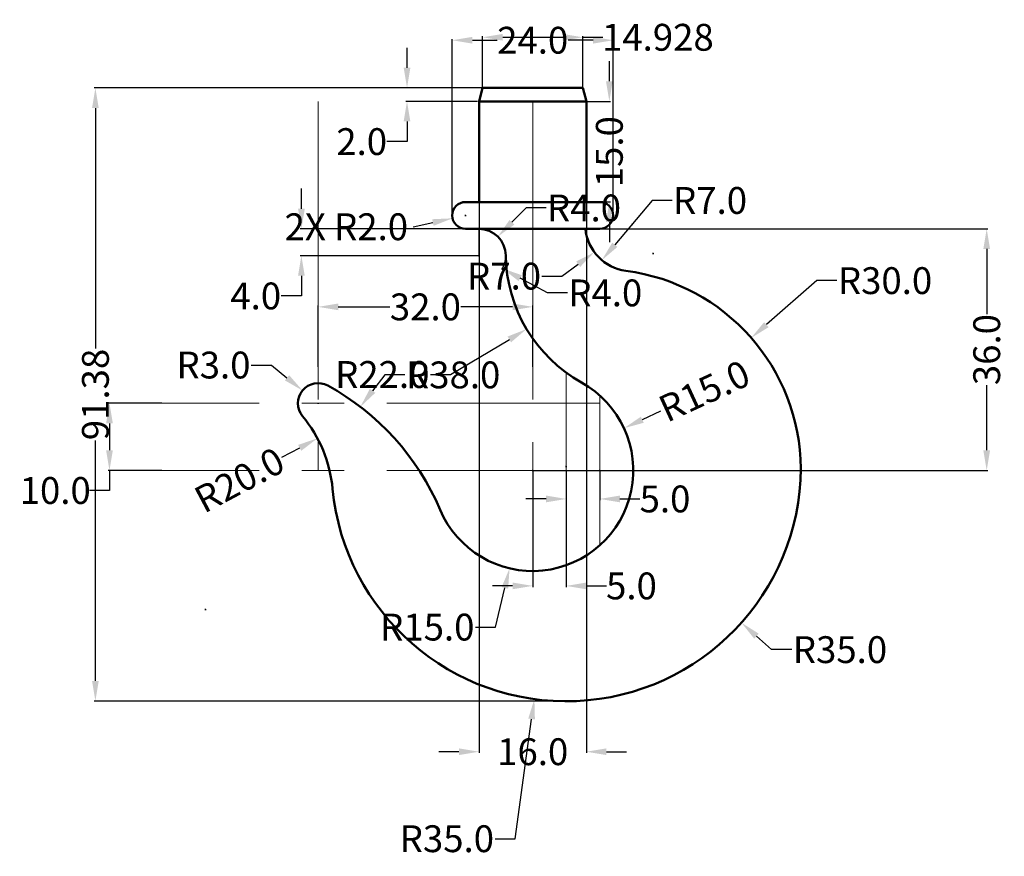
# Model space of a CAD drawing. Units: millimetres. Extents: x 373 to 520, y 647 to 772.
import ezdxf

# ---------------------------------------------------------------- set-up
doc = ezdxf.new("R2010")
doc.units = ezdxf.units.MM
doc.header["$MEASUREMENT"] = 0
doc.linetypes.add('CENTER', pattern=[50.8, 31.75, -6.35, 6.35, -6.35])
for name, color, linetype, lineweight in [('M-CNTR', 32, 'CENTER', 18), ('M-CONS', 8, 'Continuous', 13), ('M-DIMS', 2, 'Continuous', 25), ('M-OUTL', 7, 'Continuous', 50)]:
    doc.layers.add(name, color=color, linetype=linetype, lineweight=lineweight)
doc.styles.get("Standard").update_dxf_attribs({"font": 'arial.ttf'})
doc.dimstyles.get("Standard").update_dxf_attribs({"dimtxt": 4, "dimasz": 3, "dimexe": 0.18, "dimexo": 0.0625, "dimgap": 0.09, "dimtad": 0, "dimtoh": 1, "dimdec": 1, "dimzin": 0, "dimdsep": 46, "dimtxsty": 'Standard', "dimcen": 0.09, "dimadec": 0, "dimazin": 0, "dimtfac": 1, "dimtdec": 1, "dimtofl": 0, "dimtmove": 0, "dimatfit": 3, "dimfxl": 1, "dimtolj": 1, "dimtzin": 0, "dimarcsym": 0})

# ---------------------------------------------------------------- blocks, each defined once
blk = doc.blocks.new('*D1')
at = {"layer": 'Defpoints', "color": 0, "transparency": 16777216}
for p in [(482.23, 724.42), (459.65, 704.68)]:
    blk.add_point(p, dxfattribs=at)
at = {"layer": 'M-DIMS', "color": 0, "lineweight": -2, "transparency": 16777216}
for p, q in [((492, 732.96), (484.49, 726.4)), ((495, 732.96), (492, 732.96)), ((459.65, 704.59), (459.65, 704.77)), ((459.56, 704.68), (459.74, 704.68))]:
    blk.add_line(p, q, dxfattribs=at)
at = {"layer": 'M-DIMS', "color": 0, "transparency": 16777216}
blk.add_solid([(484.16, 726.77), (484.82, 726.02), (482.23, 724.42)], dxfattribs=at)
at = {"layer": 'M-DIMS', "color": 0, "transparency": 16777216, "insert": (502.19, 732.96), "char_height": 4, "attachment_point": 5}
blk.add_mtext('\\A1;R30.0', dxfattribs=at)
blk = doc.blocks.new('*D2')
at = {"layer": 'Defpoints', "color": 0, "transparency": 16777216}
for p in [(454.65, 705.26), (480.78, 681.97)]:
    blk.add_point(p, dxfattribs=at)
at = {"layer": 'M-DIMS', "color": 0, "lineweight": -2, "transparency": 16777216}
for p, q in [((454.56, 705.26), (454.74, 705.26)), ((454.65, 705.17), (454.65, 705.35)), ((485.27, 677.96), (483.01, 679.98)), ((488.27, 677.96), (485.27, 677.96))]:
    blk.add_line(p, q, dxfattribs=at)
at = {"layer": 'M-DIMS', "color": 0, "transparency": 16777216}
blk.add_solid([(483.35, 680.35), (482.68, 679.6), (480.78, 681.97)], dxfattribs=at)
at = {"layer": 'M-DIMS', "color": 0, "transparency": 16777216, "insert": (495.47, 677.96), "char_height": 4, "attachment_point": 5}
blk.add_mtext('\\A1;R35.0', dxfattribs=at)
blk = doc.blocks.new('*D3')
at = {"layer": 'Defpoints', "color": 0, "transparency": 16777216}
for p in [(441.64, 736.68), (445.15, 734.77)]:
    blk.add_point(p, dxfattribs=at)
at = {"layer": 'M-DIMS', "color": 0, "lineweight": -2, "transparency": 16777216}
for p, q in [((441.55, 736.68), (441.73, 736.68)), ((441.64, 736.59), (441.64, 736.77)), ((451.84, 731.13), (447.79, 733.33)), ((454.84, 731.13), (451.84, 731.13))]:
    blk.add_line(p, q, dxfattribs=at)
blk.add_arc((441.64, 736.68), 4, 328.9016, 359.8455, dxfattribs=at)
at = {"layer": 'M-DIMS', "color": 0, "transparency": 16777216}
blk.add_solid([(448.03, 733.77), (447.55, 732.89), (445.15, 734.77)], dxfattribs=at)
at = {"layer": 'M-DIMS', "color": 0, "transparency": 16777216, "insert": (460.47, 731.13), "char_height": 4, "attachment_point": 5}
blk.add_mtext('\\A1;R4.0', dxfattribs=at)
blk = doc.blocks.new('*D4')
at = {"layer": 'Defpoints', "color": 0, "transparency": 16777216}
for p in [(464.48, 741.36), (459.96, 736.01)]:
    blk.add_point(p, dxfattribs=at)
at = {"layer": 'M-DIMS', "color": 0, "lineweight": -2, "transparency": 16777216}
for p, q in [((467.47, 744.91), (461.9, 738.3)), ((470.47, 744.91), (467.47, 744.91))]:
    blk.add_line(p, q, dxfattribs=at)
at = {"layer": 'M-DIMS', "color": 0, "transparency": 16777216}
blk.add_solid([(461.51, 738.62), (462.28, 737.98), (459.96, 736.01)], dxfattribs=at)
at = {"layer": 'M-DIMS', "color": 0, "transparency": 16777216, "insert": (476.1, 744.91), "char_height": 4, "attachment_point": 5}
blk.add_mtext('\\A1;R7.0', dxfattribs=at)
blk = doc.blocks.new('*D5')
at = {"layer": 'Defpoints', "color": 0, "transparency": 16777216}
for p in [(441.46, 761.68), (430.91, 759.68), (441.46, 759.68)]:
    blk.add_point(p, dxfattribs=at)
at = {"layer": 'M-DIMS', "color": 0, "lineweight": -2, "transparency": 16777216}
for p, q in [((430.91, 764.68), (430.91, 767.68)), ((441.4, 761.68), (430.73, 761.68)), ((441.4, 759.68), (430.73, 759.68)), ((430.91, 756.68), (430.91, 753.68)), ((430.91, 753.68), (427.91, 753.68))]:
    blk.add_line(p, q, dxfattribs=at)
at = {"layer": 'M-DIMS', "color": 0, "transparency": 16777216}
for points in [[(430.41, 764.68), (431.41, 764.68), (430.91, 761.68)], [(430.41, 756.68), (431.41, 756.68), (430.91, 759.68)]]:
    blk.add_solid(points, dxfattribs=at)
at = {"layer": 'M-DIMS', "color": 0, "transparency": 16777216, "insert": (424.15, 753.68), "char_height": 4, "attachment_point": 5}
blk.add_mtext('\\A1;2.0', dxfattribs=at)
blk = doc.blocks.new('*D6')
at = {"layer": 'Defpoints', "color": 0, "transparency": 16777216}
for p in [(457.65, 759.68), (461.08, 759.68), (457.65, 744.68)]:
    blk.add_point(p, dxfattribs=at)
at = {"layer": 'M-DIMS', "color": 0, "lineweight": -2, "transparency": 16777216}
for p, q in [((461.08, 762.68), (461.08, 765.68)), ((457.71, 759.68), (461.26, 759.68)), ((457.71, 744.68), (461.26, 744.68)), ((461.08, 741.68), (461.08, 738.68))]:
    blk.add_line(p, q, dxfattribs=at)
at = {"layer": 'M-DIMS', "color": 0, "transparency": 16777216}
for points in [[(460.58, 762.68), (461.58, 762.68), (461.08, 759.68)], [(460.58, 741.68), (461.58, 741.68), (461.08, 744.68)]]:
    blk.add_solid(points, dxfattribs=at)
at = {"layer": 'M-DIMS', "color": 0, "transparency": 16777216, "insert": (461.08, 752.18), "char_height": 4, "attachment_point": 5, "rotation": 90}
blk.add_mtext('\\A1;15.0', dxfattribs=at)
blk = doc.blocks.new('*D7')
at = {"layer": 'Defpoints', "color": 0, "transparency": 16777216}
for p in [(461.65, 768.79), (437.65, 742.68), (461.65, 742.68)]:
    blk.add_point(p, dxfattribs=at)
at = {"layer": 'M-DIMS', "color": 0, "lineweight": -2, "transparency": 16777216}
for p, q in [((437.65, 742.74), (437.65, 768.97)), ((440.65, 768.79), (444.34, 768.79)), ((458.65, 768.79), (454.96, 768.79)), ((461.65, 742.74), (461.65, 768.97))]:
    blk.add_line(p, q, dxfattribs=at)
at = {"layer": 'M-DIMS', "color": 0, "transparency": 16777216}
for points in [[(440.65, 769.29), (440.65, 768.29), (437.65, 768.79)], [(458.65, 769.29), (458.65, 768.29), (461.65, 768.79)]]:
    blk.add_solid(points, dxfattribs=at)
at = {"layer": 'M-DIMS', "color": 0, "transparency": 16777216, "insert": (449.65, 768.79), "char_height": 4, "attachment_point": 5}
blk.add_mtext('\\A1;24.0', dxfattribs=at)
blk = doc.blocks.new('*D8')
at = {"layer": 'Defpoints', "color": 0, "transparency": 16777216}
for p in [(449.65, 704.68), (454.65, 704.68), (454.65, 687.46)]:
    blk.add_point(p, dxfattribs=at)
at = {"layer": 'M-DIMS', "color": 0, "lineweight": -2, "transparency": 16777216}
for p, q in [((449.65, 704.61), (449.65, 687.28)), ((454.65, 704.61), (454.65, 687.28)), ((446.65, 687.46), (443.65, 687.46)), ((457.65, 687.46), (460.65, 687.46))]:
    blk.add_line(p, q, dxfattribs=at)
at = {"layer": 'M-DIMS', "color": 0, "transparency": 16777216}
for points in [[(446.65, 687.96), (446.65, 686.96), (449.65, 687.46)], [(457.65, 687.96), (457.65, 686.96), (454.65, 687.46)]]:
    blk.add_solid(points, dxfattribs=at)
at = {"layer": 'M-DIMS', "color": 0, "transparency": 16777216, "insert": (464.38, 687.46), "char_height": 4, "attachment_point": 5}
blk.add_mtext('\\A1;5.0', dxfattribs=at)
blk = doc.blocks.new('*D9')
at = {"layer": 'Defpoints', "color": 0, "transparency": 16777216}
for p in [(454.65, 704.68), (459.65, 704.59), (459.65, 700.42)]:
    blk.add_point(p, dxfattribs=at)
at = {"layer": 'M-DIMS', "color": 0, "lineweight": -2, "transparency": 16777216}
for p, q in [((454.65, 704.61), (454.65, 700.24)), ((459.65, 704.52), (459.65, 700.24)), ((451.65, 700.42), (448.65, 700.42)), ((462.65, 700.42), (465.65, 700.42))]:
    blk.add_line(p, q, dxfattribs=at)
at = {"layer": 'M-DIMS', "color": 0, "transparency": 16777216}
for points in [[(451.65, 700.92), (451.65, 699.92), (454.65, 700.42)], [(462.65, 700.92), (462.65, 699.92), (459.65, 700.42)]]:
    blk.add_solid(points, dxfattribs=at)
at = {"layer": 'M-DIMS', "color": 0, "transparency": 16777216, "insert": (469.38, 700.42), "char_height": 4, "attachment_point": 5}
blk.add_mtext('\\A1;5.0', dxfattribs=at)
blk = doc.blocks.new('*D10')
at = {"layer": 'Defpoints', "color": 0, "transparency": 16777216}
for p in [(463.27, 710.97), (449.65, 704.68)]:
    blk.add_point(p, dxfattribs=at)
at = {"layer": 'M-DIMS', "color": 0, "lineweight": -2, "transparency": 16777216}
for p, q in [((468.71, 713.49), (465.99, 712.23)), ((449.65, 704.59), (449.65, 704.77)), ((449.56, 704.68), (449.74, 704.68))]:
    blk.add_line(p, q, dxfattribs=at)
at = {"layer": 'M-DIMS', "color": 0, "transparency": 16777216}
blk.add_solid([(465.78, 712.68), (466.2, 711.77), (463.27, 710.97)], dxfattribs=at)
at = {"layer": 'M-DIMS', "color": 0, "transparency": 16777216, "insert": (475.24, 716.51), "char_height": 4, "attachment_point": 5, "rotation": 24.8104}
blk.add_mtext('\\A1;R15.0', dxfattribs=at)
blk = doc.blocks.new('*D11')
at = {"layer": 'Defpoints', "color": 0, "transparency": 16777216}
for p in [(415.33, 716.58), (417.65, 714.68)]:
    blk.add_point(p, dxfattribs=at)
at = {"layer": 'M-DIMS', "color": 0, "lineweight": -2, "transparency": 16777216}
for p, q in [((407.69, 720.38), (410.69, 720.38)), ((410.69, 720.38), (413.01, 718.48)), ((417.56, 714.68), (417.74, 714.68)), ((417.65, 714.59), (417.65, 714.77))]:
    blk.add_line(p, q, dxfattribs=at)
at = {"layer": 'M-DIMS', "color": 0, "transparency": 16777216}
blk.add_solid([(413.33, 718.87), (412.69, 718.09), (415.33, 716.58)], dxfattribs=at)
at = {"layer": 'M-DIMS', "color": 0, "transparency": 16777216, "insert": (402.05, 720.38), "char_height": 4, "attachment_point": 5}
blk.add_mtext('\\A1;R3.0', dxfattribs=at)
blk = doc.blocks.new('*D12')
at = {"layer": 'Defpoints', "color": 0, "transparency": 16777216}
for p in [(417.55, 709.45), (399.9, 700.05)]:
    blk.add_point(p, dxfattribs=at)
at = {"layer": 'M-DIMS', "color": 0, "lineweight": -2, "transparency": 16777216}
blk.add_line((412.26, 706.63), (414.91, 708.04), dxfattribs=at)
at = {"layer": 'M-DIMS', "color": 0, "transparency": 16777216}
blk.add_solid([(414.67, 708.48), (415.14, 707.6), (417.55, 709.45)], dxfattribs=at)
at = {"layer": 'M-DIMS', "color": 0, "transparency": 16777216, "insert": (405.91, 703.25), "char_height": 4, "attachment_point": 5, "rotation": 28.0286}
blk.add_mtext('\\A1;R20.0', dxfattribs=at)
blk = doc.blocks.new('*D13')
at = {"layer": 'Defpoints', "color": 0, "transparency": 16777216}
for p in [(423.95, 714.15), (400.87, 683.96)]:
    blk.add_point(p, dxfattribs=at)
at = {"layer": 'M-DIMS', "color": 0, "lineweight": -2, "transparency": 16777216}
for p, q in [((427.59, 718.91), (425.77, 716.53)), ((430.59, 718.91), (427.59, 718.91)), ((400.78, 683.96), (400.96, 683.96)), ((400.87, 683.87), (400.87, 684.05))]:
    blk.add_line(p, q, dxfattribs=at)
at = {"layer": 'M-DIMS', "color": 0, "transparency": 16777216}
blk.add_solid([(425.37, 716.84), (426.17, 716.23), (423.95, 714.15)], dxfattribs=at)
at = {"layer": 'M-DIMS', "color": 0, "transparency": 16777216, "insert": (437.79, 718.91), "char_height": 4, "attachment_point": 5}
blk.add_mtext('\\A1;R38.0', dxfattribs=at)
blk = doc.blocks.new('*D14')
at = {"layer": 'Defpoints', "color": 0, "transparency": 16777216}
for p in [(394.4, 714.68), (386.54, 704.68), (394.4, 704.68)]:
    blk.add_point(p, dxfattribs=at)
at = {"layer": 'M-DIMS', "color": 0, "lineweight": -2, "transparency": 16777216}
for p, q in [((394.34, 714.68), (386.36, 714.68)), ((386.54, 711.68), (386.54, 707.68)), ((394.34, 704.68), (386.36, 704.68)), ((386.54, 704.68), (386.54, 701.68)), ((386.54, 701.68), (383.54, 701.68))]:
    blk.add_line(p, q, dxfattribs=at)
at = {"layer": 'M-DIMS', "color": 0, "transparency": 16777216}
for points in [[(386.04, 711.68), (387.04, 711.68), (386.54, 714.68)], [(386.04, 707.68), (387.04, 707.68), (386.54, 704.68)]]:
    blk.add_solid(points, dxfattribs=at)
at = {"layer": 'M-DIMS', "color": 0, "transparency": 16777216, "insert": (378.45, 701.68), "char_height": 4, "attachment_point": 5}
blk.add_mtext('\\A1;10.0', dxfattribs=at)
blk = doc.blocks.new('*D15')
at = {"layer": 'Defpoints', "color": 0, "transparency": 16777216}
for p in [(449.65, 740.68), (449.74, 704.68), (517.35, 704.68)]:
    blk.add_point(p, dxfattribs=at)
at = {"layer": 'M-DIMS', "color": 0, "lineweight": -2, "transparency": 16777216}
for p, q in [((449.71, 740.68), (517.53, 740.68)), ((517.35, 737.68), (517.35, 727.95)), ((517.35, 707.68), (517.35, 717.4)), ((449.8, 704.68), (517.53, 704.68))]:
    blk.add_line(p, q, dxfattribs=at)
at = {"layer": 'M-DIMS', "color": 0, "transparency": 16777216}
for points in [[(516.85, 737.68), (517.85, 737.68), (517.35, 740.68)], [(516.85, 707.68), (517.85, 707.68), (517.35, 704.68)]]:
    blk.add_solid(points, dxfattribs=at)
at = {"layer": 'M-DIMS', "color": 0, "transparency": 16777216, "insert": (517.35, 722.68), "char_height": 4, "attachment_point": 5, "rotation": 90}
blk.add_mtext('\\A1;36.0', dxfattribs=at)
blk = doc.blocks.new('*D16')
at = {"layer": 'Defpoints', "color": 0, "transparency": 16777216}
for p in [(417.65, 729.05), (417.65, 720.04), (449.65, 720.04)]:
    blk.add_point(p, dxfattribs=at)
at = {"layer": 'M-DIMS', "color": 0, "lineweight": -2, "transparency": 16777216}
for p, q in [((417.65, 720.11), (417.65, 729.23)), ((420.65, 729.05), (428.37, 729.05)), ((446.65, 729.05), (438.93, 729.05)), ((449.65, 720.11), (449.65, 729.23))]:
    blk.add_line(p, q, dxfattribs=at)
at = {"layer": 'M-DIMS', "color": 0, "transparency": 16777216}
for points in [[(420.65, 729.55), (420.65, 728.55), (417.65, 729.05)], [(446.65, 729.55), (446.65, 728.55), (449.65, 729.05)]]:
    blk.add_solid(points, dxfattribs=at)
at = {"layer": 'M-DIMS', "color": 0, "transparency": 16777216, "insert": (433.65, 729.05), "char_height": 4, "attachment_point": 5}
blk.add_mtext('\\A1;32.0', dxfattribs=at)
blk = doc.blocks.new('*D17')
at = {"layer": 'Defpoints', "color": 0, "transparency": 16777216}
for p in [(441.64, 740.68), (415.16, 736.68), (441.64, 736.68)]:
    blk.add_point(p, dxfattribs=at)
at = {"layer": 'M-DIMS', "color": 0, "lineweight": -2, "transparency": 16777216}
for p, q in [((415.16, 743.68), (415.16, 746.68)), ((441.57, 740.68), (414.98, 740.68)), ((441.57, 736.68), (414.98, 736.68)), ((415.16, 733.68), (415.16, 730.68)), ((415.16, 730.68), (412.16, 730.68))]:
    blk.add_line(p, q, dxfattribs=at)
at = {"layer": 'M-DIMS', "color": 0, "transparency": 16777216}
for points in [[(414.66, 743.68), (415.66, 743.68), (415.16, 740.68)], [(414.66, 733.68), (415.66, 733.68), (415.16, 736.68)]]:
    blk.add_solid(points, dxfattribs=at)
at = {"layer": 'M-DIMS', "color": 0, "transparency": 16777216, "insert": (408.35, 730.68), "char_height": 4, "attachment_point": 5}
blk.add_mtext('\\A1;4.0', dxfattribs=at)
blk = doc.blocks.new('*D18')
at = {"layer": 'Defpoints', "color": 0, "transparency": 16777216}
for p in [(442.19, 761.68), (384.44, 670.3), (456.16, 670.3)]:
    blk.add_point(p, dxfattribs=at)
at = {"layer": 'M-DIMS', "color": 0, "lineweight": -2, "transparency": 16777216}
for p, q in [((442.12, 761.68), (384.26, 761.68)), ((384.44, 758.68), (384.44, 722.83)), ((384.44, 673.3), (384.44, 709.14)), ((456.1, 670.3), (384.26, 670.3))]:
    blk.add_line(p, q, dxfattribs=at)
at = {"layer": 'M-DIMS', "color": 0, "transparency": 16777216}
for points in [[(383.94, 758.68), (384.94, 758.68), (384.44, 761.68)], [(383.94, 673.3), (384.94, 673.3), (384.44, 670.3)]]:
    blk.add_solid(points, dxfattribs=at)
at = {"layer": 'M-DIMS', "color": 0, "transparency": 16777216, "insert": (384.44, 715.99), "char_height": 4, "attachment_point": 5, "rotation": 90}
blk.add_mtext('\\A1;91.38', dxfattribs=at)
blk = doc.blocks.new('*D19')
at = {"layer": 'Defpoints', "color": 0, "transparency": 16777216}
for p in [(441.651389, 759.675544), (457.651389, 759.675544), (457.651389, 662.747036)]:
    blk.add_point(p, dxfattribs=at)
at = {"layer": 'M-DIMS', "color": 0, "lineweight": -2, "transparency": 16777216}
for p, q in [((441.651389, 759.613044), (441.651389, 662.567036)), ((457.651389, 759.613044), (457.651389, 662.567036)), ((438.651389, 662.747036), (435.651389, 662.747036)), ((460.651389, 662.747036), (463.651389, 662.747036))]:
    blk.add_line(p, q, dxfattribs=at)
at = {"layer": 'M-DIMS', "color": 0, "transparency": 16777216}
for points in [[(438.651389, 663.247036), (438.651389, 662.247036), (441.651389, 662.747036)], [(460.651389, 663.247036), (460.651389, 662.247036), (457.651389, 662.747036)]]:
    blk.add_solid(points, dxfattribs=at)
at = {"layer": 'M-DIMS', "color": 0, "transparency": 16777216, "insert": (449.651389, 662.747036), "char_height": 4, "attachment_point": 5}
blk.add_mtext('\\A1;16.0', dxfattribs=at)
blk = doc.blocks.new('*D20')
at = {"layer": 'Defpoints', "color": 0, "transparency": 16777216}
for p in [(457.12, 769.23), (442.19, 761.68), (457.12, 761.68)]:
    blk.add_point(p, dxfattribs=at)
at = {"layer": 'M-DIMS', "color": 0, "lineweight": -2, "transparency": 16777216}
for p, q in [((442.19, 761.74), (442.19, 769.41)), ((457.12, 761.74), (457.12, 769.41)), ((445.19, 769.23), (454.12, 769.23)), ((457.12, 769.23), (460.12, 769.23))]:
    blk.add_line(p, q, dxfattribs=at)
at = {"layer": 'M-DIMS', "color": 0, "transparency": 16777216}
for points in [[(445.19, 769.73), (445.19, 768.73), (442.19, 769.23)], [(454.12, 769.73), (454.12, 768.73), (457.12, 769.23)]]:
    blk.add_solid(points, dxfattribs=at)
at = {"layer": 'M-DIMS', "color": 0, "transparency": 16777216, "insert": (468.32, 769.23), "char_height": 4, "attachment_point": 5}
blk.add_mtext('\\A1;14.928', dxfattribs=at)
blk = doc.blocks.new('*D21')
at = {"layer": 'Defpoints', "color": 0, "transparency": 16777216}
for p in [(454.65, 705.26), (449.9, 670.59)]:
    blk.add_point(p, dxfattribs=at)
at = {"layer": 'M-DIMS', "color": 0, "lineweight": -2, "transparency": 16777216}
for p, q in [((454.56, 705.26), (454.74, 705.26)), ((454.65, 705.17), (454.65, 705.35)), ((447.04, 649.78), (449.49, 667.62)), ((444.04, 649.78), (447.04, 649.78))]:
    blk.add_line(p, q, dxfattribs=at)
at = {"layer": 'M-DIMS', "color": 0, "transparency": 16777216}
blk.add_solid([(448.99, 667.68), (449.98, 667.55), (449.9, 670.59)], dxfattribs=at)
at = {"layer": 'M-DIMS', "color": 0, "transparency": 16777216, "insert": (436.85, 649.78), "char_height": 4, "attachment_point": 5}
blk.add_mtext('\\A1;R35.0', dxfattribs=at)
blk = doc.blocks.new('*D22')
at = {"layer": 'Defpoints', "color": 0, "transparency": 16777216}
for p in [(449.65, 704.68), (446.2, 690.08)]:
    blk.add_point(p, dxfattribs=at)
at = {"layer": 'M-DIMS', "color": 0, "lineweight": -2, "transparency": 16777216}
for p, q in [((449.65, 704.59), (449.65, 704.77)), ((449.56, 704.68), (449.74, 704.68)), ((444.12, 681.32), (445.5, 687.16)), ((441.12, 681.32), (444.12, 681.32))]:
    blk.add_line(p, q, dxfattribs=at)
at = {"layer": 'M-DIMS', "color": 0, "transparency": 16777216}
blk.add_solid([(445.02, 687.28), (445.99, 687.04), (446.2, 690.08)], dxfattribs=at)
at = {"layer": 'M-DIMS', "color": 0, "transparency": 16777216, "insert": (433.93, 681.32), "char_height": 4, "attachment_point": 5}
blk.add_mtext('\\A1;R15.0', dxfattribs=at)
blk = doc.blocks.new('*D23')
at = {"layer": 'Defpoints', "color": 0, "transparency": 16777216}
for p in [(467.63, 737.01), (448.74, 725.74)]:
    blk.add_point(p, dxfattribs=at)
at = {"layer": 'M-DIMS', "color": 0, "lineweight": -2, "transparency": 16777216}
for p, q in [((467.63, 736.92), (467.63, 737.1)), ((467.54, 737.01), (467.72, 737.01)), ((437.41, 718.97), (446.17, 724.2)), ((434.41, 718.97), (437.41, 718.97))]:
    blk.add_line(p, q, dxfattribs=at)
at = {"layer": 'M-DIMS', "color": 0, "transparency": 16777216}
blk.add_solid([(445.91, 724.63), (446.42, 723.77), (448.74, 725.74)], dxfattribs=at)
at = {"layer": 'M-DIMS', "color": 0, "transparency": 16777216, "insert": (427.22, 718.97), "char_height": 4, "attachment_point": 5}
blk.add_mtext('\\A1;R22.0', dxfattribs=at)
blk = doc.blocks.new('*D24')
at = {"layer": 'Defpoints', "color": 0, "transparency": 16777216}
for p in [(464.48, 741.36), (458.85, 737.2)]:
    blk.add_point(p, dxfattribs=at)
at = {"layer": 'M-DIMS', "color": 0, "lineweight": -2, "transparency": 16777216}
for p, q in [((464.39, 741.36), (464.57, 741.36)), ((464.48, 741.27), (464.48, 741.45)), ((454.02, 733.63), (456.43, 735.41)), ((451.02, 733.63), (454.02, 733.63))]:
    blk.add_line(p, q, dxfattribs=at)
at = {"layer": 'M-DIMS', "color": 0, "transparency": 16777216}
blk.add_solid([(456.14, 735.82), (456.73, 735.01), (458.85, 737.2)], dxfattribs=at)
at = {"layer": 'M-DIMS', "color": 0, "transparency": 16777216, "insert": (445.38, 733.63), "char_height": 4, "attachment_point": 5}
blk.add_mtext('\\A1;R7.0', dxfattribs=at)
blk = doc.blocks.new('*D25')
at = {"layer": 'Defpoints', "color": 0, "transparency": 16777216}
for p in [(444.45, 739.52), (441.64, 736.68)]:
    blk.add_point(p, dxfattribs=at)
at = {"layer": 'M-DIMS', "color": 0, "lineweight": -2, "transparency": 16777216}
for p, q in [((448.66, 743.79), (446.55, 741.66)), ((451.66, 743.79), (448.66, 743.79)), ((441.55, 736.68), (441.73, 736.68)), ((441.64, 736.59), (441.64, 736.77))]:
    blk.add_line(p, q, dxfattribs=at)
at = {"layer": 'M-DIMS', "color": 0, "transparency": 16777216}
blk.add_solid([(446.2, 742.01), (446.91, 741.31), (444.45, 739.52)], dxfattribs=at)
at = {"layer": 'M-DIMS', "color": 0, "transparency": 16777216, "insert": (457.3, 743.79), "char_height": 4, "attachment_point": 5}
blk.add_mtext('\\A1;R4.0', dxfattribs=at)
blk = doc.blocks.new('*D26')
at = {"layer": 'Defpoints', "color": 0, "transparency": 16777216}
for p in [(437.7, 742.25), (439.65, 742.68)]:
    blk.add_point(p, dxfattribs=at)
at = {"layer": 'M-DIMS', "color": 0, "lineweight": -2, "transparency": 16777216}
for p, q in [((431.83, 740.99), (434.76, 741.62)), ((439.56, 742.68), (439.74, 742.68)), ((439.65, 742.59), (439.65, 742.77))]:
    blk.add_line(p, q, dxfattribs=at)
at = {"layer": 'M-DIMS', "color": 0, "transparency": 16777216}
blk.add_solid([(434.66, 742.11), (434.87, 741.13), (437.7, 742.25)], dxfattribs=at)
at = {"layer": 'M-DIMS', "color": 0, "transparency": 16777216, "insert": (421.86, 740.99), "char_height": 4, "attachment_point": 5}
blk.add_mtext('\\A1;2X R2.0', dxfattribs=at)

msp = doc.modelspace()

# ---------------------------------------------------------------- linework, layer by layer
at = {"layer": 'M-CNTR'}
for p, q in [((417.6514, 759.6755), (417.6514, 704.6755)), ((449.6514, 759.6755), (449.6514, 689.6755)), ((454.6514, 719.2507), (454.6514, 690.5334)), ((459.6514, 715.8559), (459.6514, 693.4952))]:
    msp.add_line(p, q, dxfattribs=at)
for points in [[(459.6514, 714.6755), (391.9947, 714.6755)], [(459.6514, 704.6755), (391.9947, 704.6755)]]:
    msp.add_lwpolyline(points, dxfattribs=at)
at = {"layer": 'M-CONS'}
msp.add_line((441.6362, 740.6755), (441.6362, 736.6755), dxfattribs=at)
at = {"layer": 'M-OUTL'}
for points in [[(441.6514, 759.6755), (457.6514, 759.6755), (457.6514, 759.6755), (457.1155, 761.6755), (442.1873, 761.6755), (441.6514, 759.6755)], [(441.6514, 759.6755), (457.6514, 759.6755), (457.6514, 744.6755), (441.6514, 744.6755)]]:
    msp.add_lwpolyline(points, close=True, dxfattribs=at)
for points in [[(439.6514, 744.6755), (459.6514, 744.6755)], [(459.6514, 740.6755), (439.6514, 740.6755)]]:
    msp.add_lwpolyline(points, dxfattribs=at)
for centre, radius, start, end in [((439.6514, 742.6755), 2, 90, 270), ((459.6514, 742.6755), 2, 270, 90), ((441.6362, 736.6755), 4, 0.74073, 90), ((464.4752, 741.3598), 7, 185.609295, 262.508911), ((467.634, 737.0117), 22, 180.74073, 240.920865), ((459.6514, 704.6755), 30, 0.540801, 82.508911), ((417.6514, 714.6755), 3, 61.342286, 219.480177), ((400.8662, 683.963), 38, 23.004419, 61.342286), ((449.6514, 704.6755), 15, 203.004419, 60.920865), ((399.899, 700.0519), 20, 5.43841, 39.480177), ((454.6514, 705.2645), 35, 185.43841, 359.499316)]:
    msp.add_arc(centre, radius, start, end, dxfattribs=at)

# ---------------------------------------------------------------- dimensions: what is measured, and where the dimension line sits
at = {"layer": 'M-DIMS'}
for base, p1, p2, override, picture, middle in [((461.6514, 768.7857), (437.6514, 742.6755), (461.6514, 742.6755), {"dimclrd": 0, "dimclre": 0, "dimclrt": 0}, '*D7', (449.6514, 768.7857)), ((457.1155, 769.2255), (442.1873, 761.6755), (457.1155, 761.6755), {"dimdec": 3, "dimlfac": 1, "dimrnd": 0, "dimzin": 0, "dimdsep": 46, "dimlunit": 2}, '*D20', (468.3242, 769.2255)), ((457.6514, 662.747), (441.6514, 759.6755), (457.6514, 759.6755), {"dimdec": 1, "dimlfac": 1, "dimrnd": 0, "dimzin": 0, "dimdsep": 46, "dimlunit": 2}, '*D19', (449.6514, 662.747)), ((417.6514, 729.0484), (449.6514, 720.0433), (417.6514, 720.0433), {"dimclrd": 0, "dimclre": 0, "dimclrt": 0}, '*D16', (433.6514, 729.0484)), ((454.6514, 687.4628), (449.6514, 704.6755), (454.6514, 704.6755), {"dimclrd": 0, "dimclre": 0, "dimclrt": 0}, '*D8', (464.3758, 687.4628)), ((459.6514, 700.4185), (454.6514, 704.6755), (459.6514, 704.5855), {"dimclrd": 0, "dimclre": 0, "dimclrt": 0}, '*D9', (469.3758, 700.4185))]:
    dim = msp.add_linear_dim(base=base, p1=p1, p2=p2, dimstyle='Standard', override=override, dxfattribs=at)
    dim.commit()
    dim.dimension.update_dxf_attribs({"geometry": picture, "text_midpoint": middle})
for base, p1, p2, override, picture, middle in [((430.9125, 759.6755), (441.4613, 761.6755), (441.4613, 759.6755), {"dimclrd": 0, "dimclre": 0, "dimclrt": 0}, '*D5', (424.154, 753.6755)), ((461.0755, 759.6755), (457.6514, 744.6755), (457.6514, 759.6755), {"dimclrd": 0, "dimclre": 0, "dimclrt": 0}, '*D6', (461.0755, 752.1755)), ((384.4447, 670.297), (442.1873, 761.6755), (456.1591, 670.297), {"dimdec": 2, "dimlfac": 1, "dimrnd": 0, "dimzin": 0, "dimdsep": 46, "dimlunit": 2}, '*D18', (384.4447, 715.9863)), ((415.1592, 736.6755), (441.6362, 740.6755), (441.6362, 736.6755), {"dimclrd": 0, "dimclre": 0, "dimclrt": 0}, '*D17', (408.3543, 730.6755)), ((517.3514, 704.6755), (449.6514, 740.6755), (449.7414, 704.6755), {"dimclrd": 0, "dimclre": 0, "dimclrt": 0}, '*D15', (517.3514, 722.6755)), ((386.5436, 704.6755), (394.3999, 714.6755), (394.3999, 704.6755), {"dimclrd": 0, "dimclre": 0, "dimclrt": 0}, '*D14', (378.4536, 701.6755))]:
    dim = msp.add_linear_dim(base=base, p1=p1, p2=p2, angle=90, dimstyle='Standard', override=override, dxfattribs=at)
    dim.commit()
    dim.dimension.update_dxf_attribs({"geometry": picture, "text_midpoint": middle})
for center, mpoint, override, picture, middle in [((464.4752, 741.3598), (459.9623, 736.0087), {"dimclrd": 0, "dimclre": 0, "dimclrt": 0}, '*D4', (476.104, 744.9055)), ((467.634, 737.0117), (448.7428, 725.7369), {"dimdec": 1, "dimlfac": 1, "dimrnd": 0, "dimzin": 0, "dimdsep": 46, "dimlunit": 2}, '*D23', (427.2157, 718.972)), ((441.6362, 736.6755), (445.1508, 734.7657), {"dimclrd": 0, "dimclre": 0, "dimclrt": 0}, '*D3', (460.4742, 731.133)), ((459.6514, 704.6755), (482.2349, 724.4236), {"dimclrd": 0, "dimclre": 0, "dimclrt": 0}, '*D1', (502.1884, 732.9593)), ((399.899, 700.0519), (417.5532, 709.4501), {"dimclrd": 0, "dimclre": 0, "dimclrt": 0}, '*D12', (405.9082, 703.2509)), ((449.6514, 704.6755), (446.1951, 690.0792), {"dimdec": 1, "dimlfac": 1, "dimrnd": 0, "dimzin": 0, "dimdsep": 46, "dimlunit": 2}, '*D22', (433.929, 681.3214)), ((454.6514, 705.2645), (449.8958, 670.5891), {"dimdec": 1, "dimlfac": 1, "dimrnd": 0, "dimzin": 0, "dimdsep": 46, "dimlunit": 2}, '*D21', (436.8501, 649.7839)), ((454.6514, 705.2645), (480.7752, 681.9719), {"dimclrd": 0, "dimclre": 0, "dimclrt": 0}, '*D2', (495.4663, 677.9607))]:
    dim = msp.add_radius_dim(center=center, mpoint=mpoint, dimstyle='Standard', override=override, dxfattribs=at)
    dim.commit()
    dim.dimension.update_dxf_attribs({"geometry": picture, "text_midpoint": middle, "dimtype": 164})
dim = msp.add_radius_dim(center=(439.6514, 742.6755), mpoint=(437.6964, 742.2535), text='2X <>', dimstyle='Standard', override={"dimdec": 1, "dimlfac": 1, "dimrnd": 0, "dimzin": 0, "dimdsep": 46, "dimlunit": 2}, dxfattribs=at)
dim.commit()
dim.dimension.update_dxf_attribs({"geometry": '*D26', "text_midpoint": (421.8616, 740.9875)})
for center, mpoint, override, picture, middle in [((441.6362, 736.6755), (444.4462, 739.5222), {"dimdec": 1, "dimlfac": 1, "dimrnd": 0, "dimzin": 0, "dimdsep": 46, "dimlunit": 2}, '*D25', (457.2997, 743.7923)), ((464.4752, 741.3598), (458.8469, 737.1977), {"dimdec": 1, "dimlfac": 1, "dimrnd": 0, "dimzin": 0, "dimdsep": 46, "dimlunit": 2}, '*D24', (445.3842, 733.6302)), ((417.6514, 714.6755), (415.3316, 716.5778), {"dimclrd": 0, "dimclre": 0, "dimclrt": 0}, '*D11', (402.0537, 720.3825)), ((400.8662, 683.963), (423.9492, 714.1487), {"dimclrd": 0, "dimclre": 0, "dimclrt": 0}, '*D13', (437.7862, 718.9149)), ((449.6514, 704.6755), (463.2669, 710.9698), {"dimclrd": 0, "dimclre": 0, "dimclrt": 0}, '*D10', (475.2416, 716.5055))]:
    dim = msp.add_radius_dim(center=center, mpoint=mpoint, dimstyle='Standard', override=override, dxfattribs=at)
    dim.commit()
    dim.dimension.update_dxf_attribs({"geometry": picture, "text_midpoint": middle})

doc.saveas('drawing.dxf')
